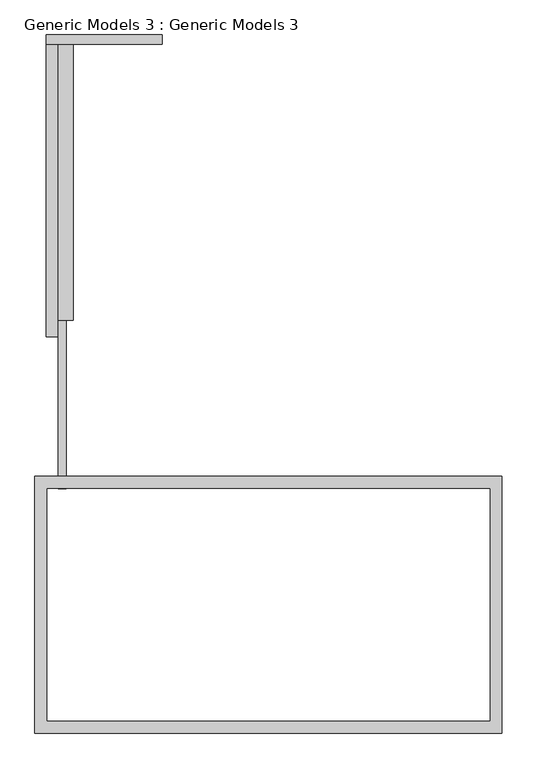
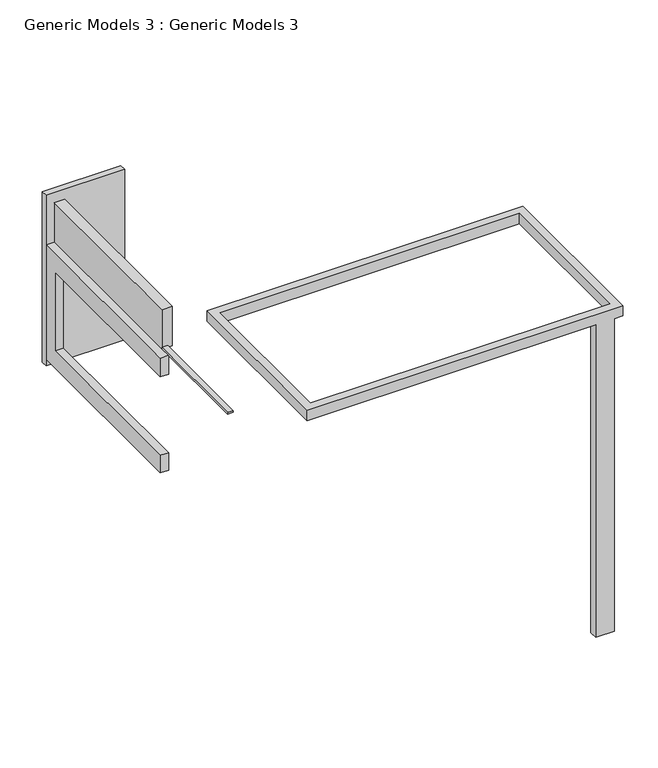
"""IFC4 building model written with IfcOpenShell, lengths in millimetres: proxy geometry, Generic Models 3 : Generic Models 3."""

from ifc_helpers import new_model, si_unit, frame, origin, place, context, project, spatial, polyline, outline, extrude, faceted_brep, source, transform, mapped, element, save


def generic_models_3_generic_models_3_0e3346f0(model_context):
    return source(origin(), model_context, "Body", "SolidModel", [
        extrude(outline(polyline([(-20112.3503587, -9529.9526331), (-20264.7503587, -9529.9526331), (-20264.7503587, -6386.2788305), (-20112.3503587, -6386.2788305), (-20112.3503587, -9529.9526331)])), frame((0.0, 0.0, 6400.8), z_axis=(0.0, 0.0, 1.0), x_axis=(1.0, 0.0, 0.0)), (0.0, 0.0, 1.0), 56.4827682),
        extrude(outline(polyline([(-19984.2998936, -6386.2788305), (-20264.7503587, -6386.2788305), (-20264.7503587, -1224.1526331), (-19984.2998936, -1224.1526331), (-19984.2998936, -6386.2788305)])), frame((0.0, 0.0, 6400.8), z_axis=(0.0, 0.0, 1.0), x_axis=(1.0, 0.0, 0.0)), (0.0, 0.0, 1.0), 1158.7368606),
        extrude(outline(polyline([(-20493.3503587, -1046.3526331), (-18321.6503587, -1046.3526331), (-18321.6503587, -1224.1526331), (-20493.3503587, -1224.1526331), (-20493.3503587, -1046.3526331)])), frame((0.0, 0.0, 2863.85), z_axis=(0.0, 0.0, 1.0), x_axis=(1.0, 0.0, 0.0)), (0.0, 0.0, 1.0), 4983.1153619),
        faceted_brep([(-12707.0553745, -14101.9526331, 0.0), (-12187.5503587, -14101.9526331, 0.0), (-12187.5503587, -14101.9526331, 9144.0), (-11958.9503587, -14101.9526331, 9144.0), (-11958.9503587, -14101.9526331, 9448.8), (-20702.9003587, -14101.9526331, 9448.8), (-20702.9003587, -14101.9526331, 9144.0), (-12707.0553745, -14101.9526331, 9144.0), (-12187.5503587, -13873.3526331, 0.0), (-12707.0553745, -13873.3526331, 0.0), (-12707.0553745, -13873.3526331, 9144.0), (-20474.3003587, -13873.3526331, 9144.0), (-20474.3003587, -13873.3526331, 9448.8), (-12187.5503587, -13873.3526331, 9448.8), (-12187.5503587, -13873.3526331, 9144.0), (-11958.9503587, -9301.3526331, 9448.8), (-20702.9003587, -9301.3526331, 9448.8), (-20474.3003587, -9529.9526331, 9448.8), (-12187.5503587, -9529.9526331, 9448.8), (-20702.9003587, -9301.3526331, 9144.0), (-11958.9503587, -9301.3526331, 9144.0), (-12187.5503587, -9529.9526331, 9144.0), (-20474.3003587, -9529.9526331, 9144.0)], [[[0, 1, 2, 3, 4, 5, 6, 7]], [[8, 9, 10, 11, 12, 13, 14]], [[9, 0, 7, 10]], [[1, 0, 9, 8]], [[1, 8, 14, 2]], [[5, 4, 15, 16], [13, 12, 17, 18]], [[6, 5, 16, 19]], [[10, 7, 6, 19, 20, 3, 2, 14, 21, 22, 11]], [[12, 11, 22, 17]], [[19, 16, 15, 20]], [[17, 22, 21, 18]], [[3, 20, 15, 4]], [[13, 18, 21, 14]]]),
        extrude(outline(polyline([(-6691.5026331, 6400.8), (-1224.1526331, 6400.8), (-1224.1526331, 3048.0), (-6691.5026331, 3048.0), (-6691.5026331, 3560.986402), (-1653.6330211, 3560.986402), (-1653.6330211, 5858.8926889), (-6691.5026331, 5858.8926889), (-6691.5026331, 6400.8)])), frame((-20493.3503587, 0.0, 0.0), z_axis=(1.0, 0.0, 0.0), x_axis=(0.0, 1.0, 0.0)), (0.0, 0.0, 1.0), 228.6),
    ])


if __name__ == "__main__":
    model = new_model("IFC4")
    model_context = context("Model", 3, world=origin())
    ifc_project = project(units=[si_unit("LENGTHUNIT", "METRE", prefix="MILLI")], contexts=[model_context])
    site = spatial("IfcSite", under=ifc_project)
    building = spatial("IfcBuilding", under=site)
    placement = place(None, origin())
    generic_models_3_generic_models_3_shape = generic_models_3_generic_models_3_0e3346f0(model_context)
    element("IfcBuildingElementProxy", 1, Name="Generic Models 3 : Generic Models 3", ObjectType="Generic Models 3 : Generic Models 3", at=placement, inside=building, context=model_context, shape_type="MappedRepresentation", body=[
        mapped(generic_models_3_generic_models_3_shape, transform((0.0, 0.0, 0.0), x_axis=(1.0, 0.0, 0.0), y_axis=(0.0, 1.0, 0.0), z_axis=(0.0, 0.0, 1.0))),
    ])
    save(model, "model.ifc")
